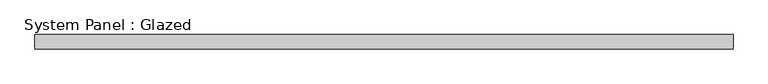
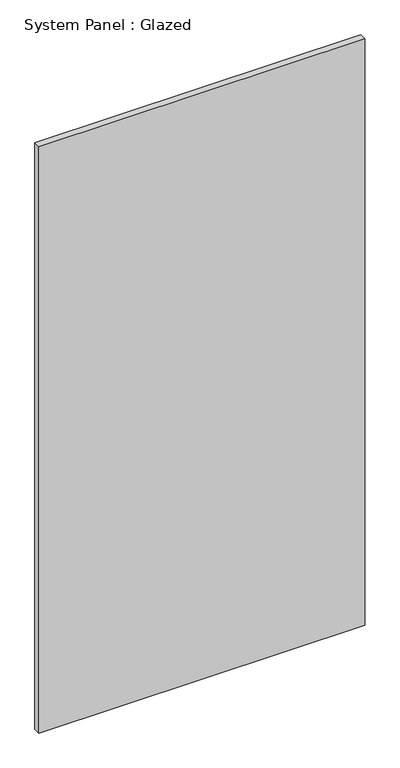
"""IFC4 building model written with IfcOpenShell, lengths in millimetres: plate geometry, System Panel : Glazed."""

from ifc_helpers import new_model, si_unit, origin, origin_with_axes, place, context, project, spatial, polyline, outline, extrude, source, transform, mapped, element, save


def system_panel_glazed_44b51bf5(model_context):
    return source(origin(), model_context, "Body", "SweptSolid", [
        extrude(outline(polyline([(615.9499999, 19.05), (-615.9499999, 19.05), (-615.9499999, 44.45), (615.9499999, 44.45), (615.9499999, 19.05)])), origin_with_axes(), (0.0, 0.0, 1.0), 2343.15),
    ])


if __name__ == "__main__":
    model = new_model("IFC4")
    model_context = context("Model", 3, world=origin())
    ifc_project = project(units=[si_unit("LENGTHUNIT", "METRE", prefix="MILLI")], contexts=[model_context])
    site = spatial("IfcSite", under=ifc_project)
    building = spatial("IfcBuilding", under=site)
    placement = place(None, origin())
    system_panel_glazed_shape = system_panel_glazed_44b51bf5(model_context)
    element("IfcPlate", 1, ObjectType="System Panel : Glazed", at=placement, inside=building, context=model_context, shape_type="MappedRepresentation", body=[
        mapped(system_panel_glazed_shape, transform((0.0, 0.0, 0.0), x_axis=(1.0, 0.0, 0.0), y_axis=(0.0, 1.0, 0.0), z_axis=(0.0, 0.0, 1.0))),
    ])
    save(model, "model.ifc")

# Revit data of these elements
# Type "System Panel : Glazed"
#   Construction Type Id = "GSP4R"
#   Analytic Construction = "1/8 in Pilkington single glazing"
#   Visual Light Transmittance = 0.9
#   Solar Heat Gain Coefficient = 0.86
#   Heat Transfer Coefficient (U) = 1.18115 BTU/(h·ft²·°F)
#   Define Thermal Properties by = 1
# Element 1 (IfcPlate, "System Panel : Glazed")
#   Materials on its faces: "Glass"
# Materials
#   "Glass": class "Glass", colour RGB 0 128 192, transparency 0.75, Description = "Soda Lime Glass", Cost = 0
